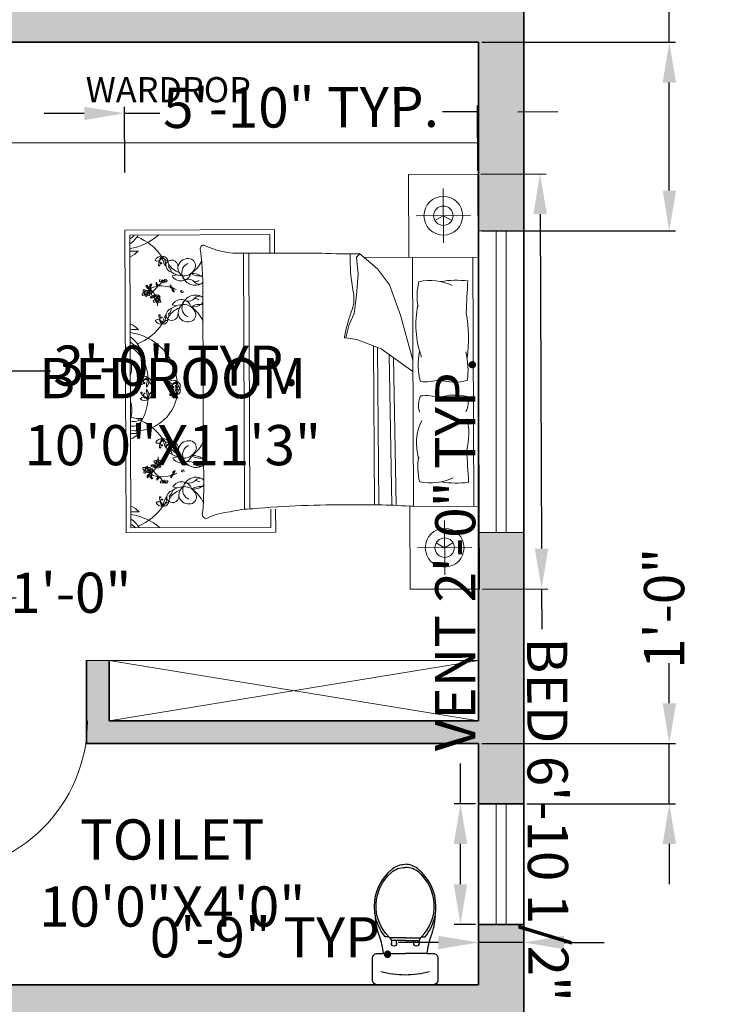
# Model space of a CAD drawing. Units: inches. Extents: x 2408 to 5087, y 2429 to 5085.
# Tile 9 of 12: x 2723 to 2864, y 2619 to 2815. Entities that reach past the tile are written whole.
import ezdxf

# ---------------------------------------------------------------- set-up
doc = ezdxf.new("R2010")
doc.units = ezdxf.units.IN
for name, color, linetype, lineweight in [('A-ANNO-DIMS', 2, 'Continuous', 18), ('A-ANNO-TEXT', 6, 'Continuous', 18), ('A-AREA-IDEN', 6, 'Continuous', 18), ('A-DOOR', 3, 'Continuous', 18), ('A-FLOR-CASE', 8, 'Continuous', 18), ('A-FLOR-FIXT', 9, 'Continuous', 18), ('A-FURN', 72, 'Continuous', 18), ('A-GLAZ', 4, 'Continuous', 18), ('A-WALL', 7, 'Continuous', 35), ('A-WALL-PATT', 252, 'Continuous', 13)]:
    doc.layers.add(name, color=color, linetype=linetype, lineweight=lineweight)
doc.layers.add('WC-Detail_dwgmodels.com', color=251, linetype='Continuous')
doc.layers.add('WC-Outline_dwgmodels.com', color=250, linetype='Continuous')
doc.styles.get("Standard").update_dxf_attribs({"font": 'arial.ttf'})
doc.dimstyles.new('ISO-25', dxfattribs={"dimtxt": 8, "dimasz": 8, "dimexe": 1.25, "dimexo": 0.625, "dimtad": 0, "dimdec": 1, "dimlunit": 4, "dimtxsty": 'Standard', "dimcen": 2.5, "dimadec": 0, "dimazin": 0, "dimtfac": 1, "dimtdec": 1, "dimtmove": 0, "dimatfit": 3, "dimfxl": 1, "dimarcsym": 0})

# ---------------------------------------------------------------- blocks, each defined once
blk = doc.blocks.new('door')
blk.add_lwpolyline([(2353.25, 2862.23), (2353.25, 2898.06), (2351.47, 2898.06), (2351.47, 2862.23), (2353.25, 2862.23)])
blk.add_arc((2353.25, 2862.23), 35.83, 90, 180)
blk = doc.blocks.new('bed')
for p, q in [((2542.13, 3205.85), (2660.24, 3205.85)), ((2553.94, 3188.29), (2553.94, 3203.72)), ((2565.75, 3205.85), (2565.75, 3173.43)), ((2636.62, 3204.33), (2565.75, 3204.33)), ((2648.43, 3188.29), (2648.43, 3203.72)), ((2561.66, 3196.01), (2546.23, 3196.01)), ((2640.72, 3196.01), (2656.15, 3196.01)), ((2565.75, 3187.18), (2636.62, 3187.18)), ((2582.16, 3183.67), (2595.04, 3187.18)), ((2598.2, 3187.18), (2591.73, 3178.18)), ((2573.55, 3180.57), (2582.16, 3183.67)), ((2636.26, 3181.07), (2593.37, 3180.46)), ((2636.3, 3182.28), (2594.25, 3181.69)), ((2569, 3177.22), (2573.55, 3180.57)), ((2591.73, 3178.18), (2589.1, 3171.24)), ((2564.7, 3172.2), (2569, 3177.22)), ((2636.2, 3176.13), (2590.88, 3175.95)), ((2636.2, 3177.35), (2591.35, 3177.17)), ((2565.65, 3171.24), (2564.7, 3172.2)), ((2570.44, 3171.72), (2565.65, 3171.24)), ((2576.42, 3171.24), (2570.44, 3171.72)), ((2581.68, 3170.52), (2576.42, 3171.24)), ((2584.79, 3169.09), (2581.68, 3170.52)), ((2589.1, 3171.24), (2588.62, 3168.13)), ((2588.62, 3168.13), (2584.79, 3169.09)), ((2557.72, 3147.95), (2564.4, 3147.95)), ((2557.72, 3105.4), (2557.72, 3147.95)), ((2637.28, 3147.95), (2643.83, 3147.95)), ((2643.83, 3147.95), (2643.83, 3105.4)), ((2564.4, 3146.58), (2559.09, 3146.58)), ((2559.09, 3146.58), (2559.09, 3106.77)), ((2642.46, 3146.58), (2637.25, 3146.58)), ((2642.46, 3106.77), (2642.46, 3146.58)), ((2637.16, 3140.58), (2564.39, 3140.58)), ((2637.27, 3139.11), (2564.39, 3139.11)), ((2625.17, 3127.51), (2577.21, 3127.51)), ((2570.73, 3118.75), (2570.47, 3120.08)), ((2578.98, 3118.75), (2579.25, 3120.08)), ((2622.57, 3118.75), (2622.31, 3120.08)), ((2630.82, 3118.75), (2631.08, 3120.08)), ((2643.83, 3105.4), (2557.72, 3105.4)), ((2559.09, 3106.77), (2642.46, 3106.77))]:
    blk.add_line(p, q)
for points in [[(2565.75, 3186.16), (2542.13, 3186.16), (2542.13, 3205.85)], [(2636.62, 3205.85), (2636.62, 3186.16), (2660.24, 3186.16), (2660.24, 3205.85)], [(2553.94, 3196.01), (2555.32, 3198.39)], [(2648.43, 3196.01), (2647.05, 3198.39)], [(2553.94, 3196.01), (2555.32, 3193.62)], [(2648.43, 3196.01), (2647.05, 3193.62)]]:
    blk.add_lwpolyline(points)
for points in [[(2572.54, 3202.91, 0.074897), (2572.68, 3195.19, -0.472817)], [(2600.63, 3194.76, 0.14099), (2600.87, 3202.63, 0.235245)], [(2605.68, 3194.76, -0.14099), (2605.44, 3202.63, -0.235245)], [(2629.84, 3202.91, -0.074897), (2629.69, 3195.19, 0.472817)], [(2564.45, 3161.38, 0.001242), (2564.39, 3138.97, -0.127202), (2562.03, 3127.8)], [(2637.13, 3141.51, 0.056112), (2637.98, 3135.02, 0.095341), (2639.64, 3128.76)]]:
    blk.add_lwpolyline(points, format="xyb")
for centre, radius in [((2553.94, 3196.01), 5.51), ((2648.43, 3196.01), 5.51), ((2553.94, 3196.01), 2.76), ((2648.43, 3196.01), 2.76), ((2577.55, 3114.47), 0.301), ((2624, 3114.47), 0.301), ((2575.59, 3111.3), 0.301), ((2625.97, 3111.3), 0.301)]:
    blk.add_circle(centre, radius)
for centre, radius, start, end in [((2637.64, 4326.92), 1125.9, 266.68521, 267.14978), ((2588.72, 3160.17), 42.84, 82.2196, 99.497), ((2597.77, 3181.81), 21.05, 81.5249, 103.96), ((2607.06, 3197.02), 5.84, 63.3437, 106.1026), ((2615.82, 3182.24), 20.76, 76.3427, 101.1841), ((2564.74, 4326.92), 1125.9, 272.85022, 273.31479), ((2587.59, 3192.09), 15.22, 155.1316, 191.7583), ((2614.79, 3192.09), 15.22, 348.2417, 24.8684), ((2586.71, 3190.81), 14.47, 354.0129, 15.8293), ((2619.6, 3190.81), 14.47, 164.1707, 185.9871), ((2585.08, 3215.54), 27.45, 258.0397, 289.2615), ((2596.2, 3209.54), 20.83, 259.8617, 283.6238), ((2607.85, 3194.98), 6.26, 245.0183, 288.5407), ((2618.79, 3203.12), 15.03, 243.8761, 286.1746), ((2576.75, 3204.29), 15.83, 255.1039, 281.0369), ((2625.62, 3204.29), 15.83, 258.9631, 284.8961), ((2848.35, 3172.75), 212.22, 176.1, 180.9282), ((2456.4, 3169.26), 108.33, 355.8294, 1.553), ((2566.72, 3214.02), 44.58, 267.4519, 281.3392), ((2577.37, 3160.89), 9.61, 66.2616, 101.3392), ((2596.82, 3212.77), 45.8, 250.1194, 259.3383), ((2588.35, 3168.04), 0.285, 268.8623, 19.7536), ((2912.96, 3165.03), 276.84, 179.1145, 184.8735), ((2563.11, 3127.88), 1.09, 183.98, 297.3412), ((2575.8, 3004.56), 122.95, 89.3433, 95.6887), ((2571.99, 3126.2), 1.42, 120.0293, 142.325), ((2571.99, 3126.2), 1.42, 44.4517, 63.558), ((2577.72, 3126.2), 1.42, 113.229, 135.5483), ((2577.72, 3126.2), 1.42, 37.675, 66.7144), ((2583.78, 3126.64), 4.89, 169.7133, 211.1782), ((2587.06, 3119.19), 8.94, 111.4941, 146.3329), ((2614.49, 3119.19), 8.94, 33.6671, 68.5059), ((2617.77, 3126.64), 4.89, 328.8218, 10.2867), ((2623.83, 3126.2), 1.42, 113.2856, 142.325), ((2623.83, 3126.2), 1.42, 44.4517, 66.7144), ((2628.78, 3012.64), 114.93, 85.2402, 91.8035), ((2629.56, 3126.2), 1.42, 106.6343, 135.5483), ((2629.56, 3126.2), 1.42, 37.675, 72.5814), ((2635.62, 3126.64), 4.89, 169.249, 211.1782), ((2638.75, 3128.16), 1.08, 246.5219, 33.8264), ((2567.86, 3123.48), 1.99, 84.4856, 181.0538), ((2562.65, 3119.19), 8.94, 33.6671, 63.2997), ((2567.25, 3122.01), 3.55, 355.2933, 76.921), ((2574.63, 3124.51), 4.56, 145.785, 184.7304), ((2565.93, 3126.64), 4.89, 328.8218, 9.1554), ((2569.72, 3125.36), 3.76, 289.2822, 29.1751), ((2574.17, 3123.35), 2.42, 131.5653, 195.1471), ((2569.15, 3124.68), 3.4, 7.436, 29.9149), ((2571.39, 3126.49), 1.77, 311.5653, 23.8354), ((2579.99, 3125.36), 3.76, 150.8249, 250.7178), ((2578.32, 3126.49), 1.77, 156.1646, 228.4347), ((2575.54, 3123.35), 2.42, 344.8529, 48.4347), ((2580.56, 3124.68), 3.4, 150.0851, 172.564), ((2575.08, 3124.51), 4.56, 355.2696, 34.215), ((2582.47, 3122.01), 3.55, 103.079, 184.7067), ((2581.85, 3123.48), 1.99, 358.9462, 95.5144), ((2619.7, 3123.48), 1.99, 84.4856, 181.0538), ((2619.08, 3122.01), 3.55, 355.2933, 76.921), ((2626.47, 3124.51), 4.56, 145.785, 184.7304), ((2621.56, 3125.36), 3.76, 289.2822, 29.1751), ((2626.01, 3123.35), 2.42, 131.5653, 195.1471), ((2620.99, 3124.68), 3.4, 7.436, 29.9149), ((2623.23, 3126.49), 1.77, 311.5653, 23.8354), ((2631.83, 3125.36), 3.76, 150.8249, 250.7178), ((2630.16, 3126.49), 1.77, 156.1646, 228.4347), ((2627.38, 3123.35), 2.42, 344.8529, 48.4347), ((2632.4, 3124.68), 3.4, 150.0851, 172.564), ((2626.92, 3124.51), 4.56, 355.2696, 34.215), ((2634.3, 3122.01), 3.55, 103.079, 184.7067), ((2638.9, 3119.19), 8.94, 113.6453, 146.3329), ((2633.69, 3123.48), 1.99, 358.9462, 95.5144), ((2568.68, 3123.2), 2.82, 174.9449, 262.8857), ((2569.79, 3124.27), 2.74, 201.5819, 291.4221), ((2569.27, 3121.29), 2.94, 299.9085, 73.1337), ((2574.63, 3124.51), 4.56, 212.7011, 216.3445), ((2571.13, 3122.53), 0.733, 257.3041, 15.1471), ((2575.17, 3121.56), 0.37, 280.4384, 100.4136), ((2580.45, 3121.29), 2.94, 106.8663, 240.0915), ((2578.59, 3122.53), 0.733, 164.8529, 282.6959), ((2575.08, 3124.51), 4.56, 323.6555, 327.2989), ((2579.93, 3124.27), 2.74, 248.5779, 338.4181), ((2581.04, 3123.2), 2.82, 277.1143, 5.0551), ((2620.51, 3123.2), 2.82, 174.9449, 262.8857), ((2621.62, 3124.27), 2.74, 201.5819, 291.4221), ((2621.1, 3121.29), 2.94, 299.9085, 73.1337), ((2626.47, 3124.51), 4.56, 212.7011, 216.3445), ((2622.96, 3122.53), 0.733, 257.3041, 15.1471), ((2626.38, 3121.56), 0.37, 79.5864, 259.5616), ((2632.29, 3121.29), 2.94, 106.8663, 240.0915), ((2630.43, 3122.53), 0.733, 164.8529, 282.6959), ((2626.92, 3124.51), 4.56, 323.6555, 327.2989), ((2631.76, 3124.27), 2.74, 248.5779, 338.4181), ((2632.87, 3123.2), 2.82, 277.1143, 5.0551), ((2568.03, 3118.65), 1.77, 80.264, 250.8688), ((2564.51, 3122.55), 5.58, 301.2614, 341.7045), ((2568.19, 3123.83), 3.43, 272.3591, 324.0401), ((2564.46, 3122.1), 6.34, 326.2883, 356.5076), ((2583.38, 3115.47), 9.78, 153.0032, 159.8941), ((2574.57, 3118.82), 0.241, 84.3784, 186.0543), ((2574.08, 3120.88), 1.9, 285.5129, 293.6099), ((2575.32, 3118.75), 0.62, 87.3579, 140.4944), ((2573.89, 3120.53), 1.87, 301.164, 321.5612), ((2575.2, 3121.41), 0.228, 102.7051, 280.4384), ((2572.37, 3120.86), 3.33, 324.6898, 333.4936), ((2581.53, 3123.83), 3.43, 215.9599, 267.6409), ((2585.25, 3122.1), 6.34, 183.4924, 213.7117), ((2585.2, 3122.55), 5.58, 198.2955, 238.7386), ((2581.69, 3118.65), 1.77, 289.1312, 99.736), ((2602.11, 3104.69), 15.42, 94.4623, 172.255), ((2602.17, 3118.92), 1.71, 137.7873, 219.1145), ((2600.23, 3118.97), 1.29, 298.5391, 58.3627), ((2602.13, 3119.71), 1.28, 63.0274, 163.8037), ((2600.84, 3122.7), 2.63, 271.4585, 315.3727), ((2601.91, 3117.85), 2.44, 45.5411, 114.3101), ((2604.13, 3130.37), 10.79, 252.593, 267.2582), ((2602.17, 3120.02), 1.26, 177.7585, 283.852), ((2604.6, 3121.34), 3.9, 198.9159, 238.011), ((2603.58, 3117.85), 2.44, 65.6899, 134.4589), ((2601.35, 3130.37), 10.79, 272.7418, 287.407), ((2602.43, 3118.96), 0.167, 283.852, 219.9245), ((2603.35, 3119.71), 1.28, 16.1963, 116.9726), ((2604.65, 3122.7), 2.63, 224.6273, 268.5415), ((2603.04, 3119.02), 0.101, 320.1909, 256.0209), ((2600.89, 3121.34), 3.9, 301.989, 341.0841), ((2603.32, 3120.02), 1.26, 256.148, 2.2415), ((2605.26, 3118.97), 1.29, 121.6373, 241.4609), ((2603.32, 3118.92), 1.71, 320.8855, 42.2127), ((2602.88, 3108.26), 11.94, 352.8636, 81.8197), ((2619.87, 3118.65), 1.77, 80.264, 250.8688), ((2616.35, 3122.55), 5.58, 301.2614, 341.7045), ((2620.02, 3123.83), 3.43, 272.3591, 324.0401), ((2616.3, 3122.1), 6.34, 326.2883, 356.5076), ((2627.67, 3120.53), 1.87, 218.4388, 238.836), ((2626.23, 3118.75), 0.62, 39.5056, 92.6421), ((2629.18, 3120.86), 3.33, 206.5064, 215.3102), ((2626.36, 3121.41), 0.228, 259.5616, 77.2949), ((2627.47, 3120.88), 1.9, 246.3901, 254.4871), ((2618.17, 3115.47), 9.78, 20.1059, 26.9968), ((2626.99, 3118.82), 0.241, 353.9457, 95.6216), ((2633.36, 3123.83), 3.43, 215.9599, 267.6409), ((2637.09, 3122.1), 6.34, 183.4924, 213.7117), ((2637.04, 3122.55), 5.58, 198.2955, 238.7386), ((2633.52, 3118.65), 1.77, 289.1312, 99.736), ((2566.53, 3116.2), 1.28, 92.9516, 193.728), ((2563.91, 3118.15), 2.63, 301.3827, 345.2969), ((2567.26, 3114.47), 2.44, 75.4653, 144.2343), ((2562.95, 3126.43), 10.79, 282.5173, 297.1824), ((2567.66, 3116.73), 1.09, 63.9755, 143.2681), ((2567.6, 3119.18), 2.21, 265.969, 344.3045), ((2569.99, 3116.24), 2.36, 96.1662, 141.5825), ((2572.14, 3116.72), 0.502, 101.5637, 142.6358), ((2571.72, 3116.26), 0.301, 273.2768, 86.7232), ((2572.07, 3116.54), 0.287, 91.1081, 181.8675), ((2572.38, 3115.96), 0.622, 80.3487, 133.6538), ((2571.74, 3117.11), 0.723, 288.7263, 352.5032), ((2572.26, 3115.32), 0.985, 83.0852, 105.7171), ((2572.23, 3117.08), 0.232, 345.2356, 144.9248), ((2572.44, 3116.32), 0.259, 317.6792, 80.3487), ((2573.89, 3117.9), 0.62, 101.3256, 154.4621), ((2573, 3120), 1.87, 280.2588, 300.656), ((2573.43, 3121.49), 3.33, 268.3264, 277.1302), ((2583.38, 3115.47), 9.78, 163.5842, 183.8277), ((2572.6, 3120), 1.9, 308.2101, 316.3071), ((2573.76, 3118.75), 0.567, 278.3432, 4.2869), ((2573.45, 3119.25), 0.99, 300.656, 332.6341), ((2574.19, 3118.59), 0.241, 55.7657, 157.4417), ((2574.34, 3119.78), 0.99, 269.1859, 301.164), ((2574.63, 3119.27), 0.567, 237.5332, 323.4768), ((2579.73, 3116.24), 2.36, 38.4175, 83.8338), ((2582.11, 3119.18), 2.21, 195.6955, 274.031), ((2582.05, 3116.73), 1.09, 36.7319, 116.0245), ((2582.45, 3114.47), 2.44, 35.7657, 104.5347), ((2586.77, 3126.43), 10.79, 242.8176, 257.4827), ((2583.19, 3116.2), 1.28, 346.272, 87.0484), ((2585.8, 3118.15), 2.63, 194.7031, 238.6173), ((2602.63, 3118.19), 0.192, 238.011, 71.5592), ((2602.66, 3118.28), 0.093, 71.5592, 188.0167), ((2602.86, 3118.19), 0.192, 108.4408, 301.989), ((2602.83, 3118.28), 0.093, 351.9833, 108.4408), ((2618.36, 3116.2), 1.28, 92.9516, 193.728), ((2615.75, 3118.15), 2.63, 301.3827, 345.2969), ((2619.1, 3114.47), 2.44, 75.4653, 144.2343), ((2614.78, 3126.43), 10.79, 282.5173, 297.1824), ((2619.5, 3116.73), 1.09, 63.9755, 143.2681), ((2619.44, 3119.18), 2.21, 265.969, 344.3045), ((2621.82, 3116.24), 2.36, 96.1662, 141.5825), ((2626.92, 3119.27), 0.567, 216.5232, 302.4668), ((2627.21, 3119.78), 0.99, 238.836, 270.8141), ((2627.79, 3118.75), 0.567, 175.7131, 261.6568), ((2627.36, 3118.59), 0.241, 22.5583, 124.2343), ((2628.1, 3119.25), 0.99, 207.3659, 239.344), ((2618.17, 3115.47), 9.78, 356.1723, 16.4158), ((2628.96, 3120), 1.9, 223.6929, 231.7899), ((2628.55, 3120), 1.87, 239.344, 259.7412), ((2628.12, 3121.49), 3.33, 262.8698, 271.6736), ((2627.66, 3117.9), 0.62, 25.5379, 78.6744), ((2629.11, 3116.32), 0.259, 99.6513, 222.3208), ((2629.17, 3115.96), 0.622, 46.3462, 99.6513), ((2629.32, 3117.08), 0.232, 35.0752, 194.7644), ((2629.82, 3117.11), 0.723, 187.4968, 251.2737), ((2629.29, 3115.32), 0.985, 74.2829, 96.9148), ((2629.48, 3116.54), 0.287, 358.1325, 88.8919), ((2629.41, 3116.72), 0.502, 37.3642, 78.4363), ((2629.83, 3116.26), 0.301, 93.2768, 266.7232), ((2633.95, 3119.18), 2.21, 195.6955, 274.031), ((2631.56, 3116.24), 2.36, 38.4175, 83.8338), ((2633.89, 3116.73), 1.09, 36.7319, 116.0245), ((2634.29, 3114.47), 2.44, 35.7657, 104.5347), ((2638.61, 3126.43), 10.79, 242.8176, 257.4827), ((2637.64, 3118.15), 2.63, 194.7031, 238.6173), ((2635.02, 3116.2), 1.28, 346.272, 87.0484), ((2547.61, 3104.69), 15.42, 7.745, 41.8856), ((2574, 3103.17), 15.42, 124.3865, 158.5908), ((2566.96, 3115.53), 1.71, 167.7115, 249.0387), ((2565.25, 3114.61), 1.29, 328.4633, 88.2869), ((2567.85, 3118.83), 3.9, 228.8402, 267.9352), ((2566.4, 3116.48), 1.26, 207.6827, 313.7762), ((2567.16, 3115.69), 0.167, 313.7762, 249.7183), ((2567.7, 3115.22), 0.093, 101.4834, 217.9409), ((2567.72, 3115.13), 0.192, 267.9352, 101.4834), ((2572.13, 3115.7), 0.497, 217.7621, 259.0403), ((2572.67, 3116.36), 0.913, 203.4276, 227.6104), ((2572.27, 3116.48), 0.492, 229.7889, 317.6792), ((2571.71, 3115.43), 0.699, 355.053, 68.3618), ((2572.18, 3115.39), 0.231, 232.4737, 355.053), ((2565.44, 3107.15), 11.21, 43.1541, 52.0459), ((2573.19, 3113.92), 0.62, 101.3256, 154.4621), ((2572.3, 3116.03), 1.87, 280.2588, 300.656), ((2572.73, 3117.52), 3.33, 268.3264, 277.1302), ((2571.89, 3116.02), 1.9, 308.2101, 316.3071), ((2573.06, 3114.77), 0.567, 278.3432, 4.2869), ((2572.74, 3115.27), 0.99, 300.656, 332.6341), ((2573.49, 3114.62), 0.241, 55.7657, 157.4417), ((2578.51, 3115.22), 4.9, 184.756, 209.2041), ((2585.57, 3125.67), 16.14, 222.2412, 232.1744), ((2579.01, 3108.71), 5.88, 120.544, 139.818), ((2575.98, 3114.61), 0.833, 272.8499, 356.1226), ((2575.25, 3114.91), 1.37, 304.5369, 16.3699), ((2575.39, 3114.28), 0.807, 321.7607, 7.9252), ((2575.56, 3113.13), 0.807, 8.7227, 54.8872), ((2575.61, 3112.48), 1.37, 0.278, 72.111), ((2577.15, 3114.53), 0.97, 127.3105, 187.9252), ((2576.22, 3112.98), 0.833, 20.5253, 88.5375), ((2575.82, 3114.64), 0.996, 355.0106, 41.658), ((2576.92, 3113.9), 0.298, 148.0499, 225.6268), ((2579.01, 3108.71), 5.88, 113.0501, 113.8477), ((2577.47, 3113.56), 0.948, 104.7558, 148.0499), ((2576.94, 3114.24), 0.594, 247.4086, 351.4386), ((2577.22, 3114.89), 0.41, 126.1046, 271.4281), ((2577.18, 3115), 0.295, 353.7526, 131.7054), ((2577.11, 3114.21), 0.199, 262.906, 7.132), ((2576.9, 3114.65), 0.414, 0.0645, 61.1507), ((2577, 3115), 0.473, 311.8413, 355.7877), ((2577.97, 3114.93), 0.502, 101.5637, 176.365), ((2577.96, 3113.91), 0.497, 151.2196, 259.0403), ((2577.9, 3114.75), 0.287, 91.1081, 181.8675), ((2578.5, 3114.57), 0.913, 203.4276, 227.6104), ((2578.21, 3114.17), 0.622, 80.3487, 133.6538), ((2578.1, 3114.69), 0.492, 229.7889, 317.6792), ((2577.57, 3115.33), 0.723, 288.7263, 352.5032), ((2577.54, 3113.65), 0.699, 355.053, 68.3618), ((2578.09, 3113.53), 0.985, 83.0852, 105.7171), ((2578.06, 3115.29), 0.232, 345.2356, 144.9248), ((2578.01, 3113.61), 0.231, 232.4737, 355.053), ((2578.27, 3114.53), 0.259, 317.6792, 80.3487), ((2579.01, 3108.71), 5.88, 87.1071, 94.7585), ((2582, 3115.13), 0.192, 78.5166, 272.0648), ((2581.86, 3118.83), 3.9, 272.0648, 311.1598), ((2582.02, 3115.22), 0.093, 322.0591, 78.5166), ((2583.31, 3116.48), 1.26, 226.2238, 332.3173), ((2582.57, 3115.76), 0.101, 290.2667, 226.2271), ((2584.47, 3114.61), 1.29, 91.7131, 211.5367), ((2582.76, 3115.53), 1.71, 290.9613, 12.2885), ((2575.72, 3103.17), 15.42, 21.4092, 55.6135), ((2625.83, 3103.17), 15.42, 124.3865, 158.5908), ((2618.79, 3115.53), 1.71, 167.7115, 249.0387), ((2618.24, 3116.48), 1.26, 207.6827, 313.7762), ((2619.69, 3118.83), 3.9, 228.8402, 267.9352), ((2617.08, 3114.61), 1.29, 328.4633, 88.2869), ((2619, 3115.69), 0.167, 313.7762, 249.7183), ((2619.54, 3115.22), 0.093, 101.4834, 217.9409), ((2619.56, 3115.13), 0.192, 267.9352, 101.4834), ((2622.54, 3108.71), 5.88, 85.2415, 92.8929), ((2623.28, 3114.53), 0.259, 99.6513, 222.3208), ((2623.45, 3114.69), 0.492, 222.3208, 310.2111), ((2623.34, 3114.17), 0.622, 46.3462, 99.6513), ((2623.49, 3115.29), 0.232, 35.0752, 194.7644), ((2623.98, 3115.33), 0.723, 187.4968, 251.2737), ((2624.01, 3113.65), 0.699, 111.6382, 184.947), ((2623.54, 3113.61), 0.231, 184.947, 307.5263), ((2623.46, 3113.53), 0.985, 74.2829, 96.9148), ((2623.65, 3114.75), 0.287, 358.1325, 88.8919), ((2623.05, 3114.57), 0.913, 312.3896, 336.5724), ((2623.58, 3114.93), 0.502, 3.635, 78.4363), ((2623.59, 3113.91), 0.497, 280.9597, 28.7804), ((2624.61, 3114.24), 0.594, 188.5614, 292.5914), ((2624.38, 3115), 0.295, 48.2946, 186.2474), ((2624.55, 3115), 0.473, 184.2123, 228.1587), ((2624.65, 3114.65), 0.414, 118.8493, 179.9355), ((2624.44, 3114.21), 0.199, 172.868, 277.094), ((2624.33, 3114.89), 0.41, 268.5719, 53.8954), ((2624.08, 3113.56), 0.948, 31.9501, 75.2442), ((2625.33, 3112.98), 0.833, 91.4625, 159.4747), ((2625.94, 3112.48), 1.37, 107.889, 179.722), ((2625.73, 3114.64), 0.996, 138.342, 184.9894), ((2625.57, 3114.61), 0.833, 183.8774, 267.1501), ((2622.54, 3108.71), 5.88, 66.1523, 66.9499), ((2624.63, 3113.9), 0.298, 314.3732, 31.9501), ((2626.3, 3114.91), 1.37, 163.6301, 235.4631), ((2624.4, 3114.53), 0.97, 352.0748, 52.6895), ((2625.99, 3113.13), 0.807, 125.1128, 171.2773), ((2626.16, 3114.28), 0.807, 172.0748, 218.2393), ((2622.54, 3108.71), 5.88, 40.182, 59.456), ((2615.98, 3125.67), 16.14, 307.8256, 317.7588), ((2623.04, 3115.22), 4.9, 330.7959, 355.244), ((2636.11, 3107.15), 11.21, 127.9541, 136.8459), ((2628.06, 3114.62), 0.241, 22.5583, 124.2343), ((2628.49, 3114.77), 0.567, 175.7131, 261.6568), ((2628.81, 3115.27), 0.99, 207.3659, 239.344), ((2629.66, 3116.02), 1.9, 223.6929, 231.7899), ((2629.26, 3116.03), 1.87, 239.344, 259.7412), ((2628.83, 3117.52), 3.33, 262.8698, 271.6736), ((2628.36, 3113.92), 0.62, 25.5379, 78.6744), ((2629.29, 3116.48), 0.492, 222.3208, 310.2111), ((2629.84, 3115.43), 0.699, 111.6382, 184.947), ((2629.37, 3115.39), 0.231, 184.947, 307.5263), ((2628.88, 3116.36), 0.913, 312.3896, 336.5724), ((2629.42, 3115.7), 0.497, 280.9597, 322.2379), ((2633.83, 3115.13), 0.192, 78.5166, 272.0648), ((2633.7, 3118.83), 3.9, 272.0648, 311.1598), ((2633.85, 3115.22), 0.093, 322.0591, 78.5166), ((2635.15, 3116.48), 1.26, 226.2238, 332.3173), ((2634.41, 3115.76), 0.101, 290.2667, 226.2271), ((2636.31, 3114.61), 1.29, 91.7131, 211.5367), ((2634.6, 3115.53), 1.71, 290.9613, 12.2885), ((2627.56, 3103.17), 15.42, 21.4092, 55.6135), ((2653.94, 3104.69), 15.42, 138.1144, 172.255), ((2573.4, 3112.83), 0.336, 146.8636, 236.9021), ((2578.13, 3120.23), 8.79, 235.1882, 238.8844), ((2573.97, 3113.32), 0.909, 199.4799, 267.6828), ((2573.87, 3112.98), 0.783, 212.8155, 277.3992), ((2573.42, 3112.45), 0.909, 266.9701, 338.2913), ((2568.62, 3118.94), 8.79, 302.6784, 306.3746), ((2573.65, 3111.74), 0.336, 214.3538, 304.3923), ((2573.77, 3113.01), 0.348, 238.8844, 314.2646), ((2573.7, 3112.23), 0.783, 280.3057, 17.1958), ((2573.63, 3112.15), 0.348, 306.3746, 21.7548), ((2574.2, 3112.37), 0.262, 19.3605, 201.7548), ((2574.2, 3112.57), 0.262, 311.8703, 134.2646), ((2579.13, 3110.18), 5.24, 153.7819, 158.2913), ((2574.96, 3113.76), 1.37, 247.2305, 319.0635), ((2574.51, 3113.3), 0.807, 264.4544, 310.6188), ((2578.51, 3115.22), 4.9, 214.0033, 222.4917), ((2575.1, 3112.98), 0.833, 218.3208, 298.8162), ((2574.95, 3110.73), 0.298, 148.0499, 225.6268), ((2575.51, 3110.39), 0.948, 104.7558, 148.0499), ((2574.97, 3111.07), 0.594, 247.4086, 351.4386), ((2575.25, 3111.72), 0.41, 126.1046, 271.4281), ((2575.21, 3111.83), 0.295, 353.7526, 131.7054), ((2575.66, 3111.95), 0.97, 70.0041, 130.6188), ((2575.14, 3111.04), 0.199, 262.906, 7.132), ((2574.93, 3111.48), 0.414, 0.0645, 61.1507), ((2575.03, 3111.83), 0.473, 311.8413, 355.7877), ((2575.04, 3113.13), 0.996, 297.7043, 344.3516), ((2576, 3111.76), 0.502, 101.5637, 176.365), ((2576, 3110.74), 0.497, 151.2196, 259.0403), ((2575.94, 3111.58), 0.287, 91.1081, 181.8675), ((2576.53, 3111.4), 0.913, 203.4276, 227.6104), ((2576.24, 3111), 0.622, 80.3487, 133.6538), ((2576.13, 3111.52), 0.492, 229.7889, 317.6792), ((2575.6, 3112.16), 0.723, 288.7263, 352.5032), ((2575.58, 3110.48), 0.699, 355.053, 68.3618), ((2576.12, 3110.36), 0.985, 83.0852, 105.7171), ((2576.09, 3112.12), 0.232, 345.2356, 144.9248), ((2576.3, 3111.36), 0.259, 317.6792, 80.3487), ((2577.32, 3113.39), 0.97, 188.7227, 249.3375), ((2576.08, 3112.91), 0.996, 334.9899, 21.6373), ((2600.93, 3096.43), 15.42, 94.4623, 117.4146), ((2600.99, 3110.66), 1.71, 137.7873, 219.1145), ((2599.05, 3110.71), 1.29, 298.5391, 58.3627), ((2600.99, 3111.76), 1.26, 177.7585, 283.852), ((2600.95, 3111.45), 1.28, 63.0274, 163.8037), ((2599.66, 3114.44), 2.63, 271.4585, 315.3727), ((2600.73, 3109.59), 2.44, 45.5411, 114.3101), ((2603.42, 3113.07), 3.9, 198.9159, 238.011), ((2602.95, 3122.11), 10.79, 252.593, 267.2582), ((2601.25, 3110.7), 0.167, 283.852, 219.9245), ((2604.76, 3109.59), 2.44, 65.6899, 134.4589), ((2602.54, 3122.11), 10.79, 272.7418, 287.407), ((2604.54, 3111.45), 1.28, 16.1963, 116.9726), ((2605.83, 3114.44), 2.63, 224.6273, 268.5415), ((2604.22, 3110.76), 0.101, 320.1909, 256.0209), ((2602.07, 3113.07), 3.9, 301.989, 341.0841), ((2604.5, 3111.76), 1.26, 256.148, 2.2415), ((2606.44, 3110.71), 1.29, 121.6373, 241.4609), ((2604.5, 3110.66), 1.71, 320.8855, 42.2127), ((2604.56, 3096.43), 15.42, 62.5854, 85.5377), ((2625.48, 3112.91), 0.996, 158.3627, 205.0101), ((2624.23, 3113.39), 0.97, 290.6625, 351.2773), ((2625.25, 3111.36), 0.259, 99.6513, 222.3208), ((2625.42, 3111.52), 0.492, 222.3208, 310.2111), ((2625.31, 3111), 0.622, 46.3462, 99.6513), ((2625.46, 3112.12), 0.232, 35.0752, 194.7644), ((2625.95, 3112.16), 0.723, 187.4968, 251.2737), ((2625.98, 3110.48), 0.699, 111.6382, 184.947), ((2625.43, 3110.36), 0.985, 74.2829, 96.9148), ((2625.89, 3111.95), 0.97, 49.3812, 109.9959), ((2626.59, 3113.76), 1.37, 220.9365, 292.7695), ((2626.52, 3113.13), 0.996, 195.6484, 242.2957), ((2625.62, 3111.58), 0.287, 358.1325, 88.8919), ((2625.02, 3111.4), 0.913, 312.3896, 336.5724), ((2625.55, 3111.76), 0.502, 3.635, 78.4363), ((2625.56, 3110.74), 0.497, 280.9597, 28.7804), ((2626.58, 3111.07), 0.594, 188.5614, 292.5914), ((2626.45, 3112.98), 0.833, 241.1838, 321.6792), ((2626.34, 3111.83), 0.295, 48.2946, 186.2474), ((2626.52, 3111.83), 0.473, 184.2123, 228.1587), ((2626.62, 3111.48), 0.414, 118.8493, 179.9355), ((2626.41, 3111.04), 0.199, 172.868, 277.094), ((2626.3, 3111.72), 0.41, 268.5719, 53.8954), ((2626.05, 3110.39), 0.948, 31.9501, 75.2442), ((2627.04, 3113.3), 0.807, 229.3812, 275.5456), ((2623.04, 3115.22), 4.9, 317.5083, 325.9967), ((2626.6, 3110.73), 0.298, 314.3732, 31.9501), ((2627.86, 3112.23), 0.783, 162.8042, 259.6943), ((2627.35, 3112.57), 0.262, 45.7354, 228.1297), ((2627.36, 3112.37), 0.262, 338.2452, 160.6395), ((2622.42, 3110.18), 5.24, 21.7087, 26.2181), ((2628.13, 3112.45), 0.909, 201.7087, 273.0299), ((2627.78, 3113.01), 0.348, 225.7354, 301.1156), ((2627.92, 3112.15), 0.348, 158.2452, 233.6254), ((2627.68, 3112.98), 0.783, 262.6008, 327.1845), ((2627.58, 3113.32), 0.909, 272.3172, 340.5201), ((2632.93, 3118.94), 8.79, 233.6254, 237.3216), ((2627.91, 3111.74), 0.336, 235.6077, 325.6462), ((2623.42, 3120.23), 8.79, 301.1156, 304.8118), ((2628.15, 3112.83), 0.336, 303.0979, 33.1364), ((2555.35, 3102.63), 7.52, 33.4617, 60.1116), ((2552.64, 3101.23), 9.37, 36.3036, 46.4814), ((2559.56, 3104.37), 6.27, 22.5547, 48.9546), ((2542.38, 3107.74), 21.34, 357.4081, 3.6519), ((2576.04, 3110.44), 0.231, 232.4737, 355.053), ((2590.16, 3104.37), 6.27, 131.0454, 157.4453), ((2607.34, 3107.74), 21.34, 176.3481, 182.5919), ((2594.37, 3102.63), 7.52, 91.272, 146.5383), ((2597.07, 3101.23), 9.37, 107.8504, 143.6964), ((2601.99, 3098.59), 13.93, 124.0123, 144.053), ((2601.45, 3109.93), 0.192, 238.011, 71.5592), ((2601.48, 3110.02), 0.093, 71.5592, 188.0167), ((2604.04, 3109.93), 0.192, 108.4408, 301.989), ((2604.01, 3110.02), 0.093, 351.9833, 108.4408), ((2604.43, 3109.35), 6.91, 338.117, 6.6195), ((2610.76, 3107.42), 2.77, 346.3898, 79.0739), ((2608.68, 3107.8), 3.5, 342.8609, 41.9049), ((2594.21, 3107.74), 21.34, 357.4081, 3.6519), ((2611.39, 3104.37), 6.27, 22.5547, 48.9546), ((2625.51, 3110.44), 0.231, 184.947, 307.5263), ((2642, 3104.37), 6.27, 131.0454, 157.4453), ((2659.17, 3107.74), 21.34, 176.3481, 182.5919), ((2646.21, 3102.63), 7.52, 119.8884, 146.5383), ((2648.91, 3101.23), 9.37, 133.5186, 143.6964), ((2596.61, 3098.66), 8.48, 73.5431, 107.0202), ((2599.97, 3094.29), 12.54, 94.3787, 95.6357), ((2606.58, 3085.7), 22.41, 109.7217, 109.9028), ((2608.88, 3098.66), 8.48, 72.9798, 106.4569), ((2605.52, 3094.29), 12.54, 84.3643, 85.6213), ((2598.91, 3085.7), 22.41, 70.0972, 70.2783)]:
    blk.add_arc(centre, radius, start, end)
blk = doc.blocks.new('pan')
at = {"layer": 'WC-Detail_dwgmodels.com'}
for p, q in [((2600.67, 3096.11), (2600.67, 3096.83)), ((2601.96, 3096.83), (2601.96, 3096.11)), ((2606.1, 3096.83), (2606.1, 3096.11)), ((2607.39, 3096.11), (2607.39, 3096.83)), ((2600.31, 3095.45), (2600.67, 3096.11)), ((2601.96, 3096.11), (2600.67, 3096.11)), ((2604.03, 3096.11), (2601.96, 3096.11)), ((2604.03, 3096.11), (2606.1, 3096.11)), ((2606.1, 3096.11), (2607.39, 3096.11)), ((2607.75, 3095.45), (2607.39, 3096.11))]:
    blk.add_line(p, q, dxfattribs=at)
for points in [[(2600.04, 3095.18, 0.434217), (2600.67, 3079.55, 0.182634), (2604.03, 3078.32, 2.693815)], [(2599.14, 3095.18, 0.094048), (2597.09, 3091.32, 0.16845)], [(2600.04, 3095.18), (2599.14, 3095.18, 0.416606)], [(2600.31, 3095.45, 0.008985), (2600.04, 3095.18, 0.182634)], [(2604.03, 3095.45), (2600.31, 3095.45, 0.008985)], [(2604.03, 3095.45), (2607.75, 3095.45, -0.444938)], [(2608.02, 3095.18, -0.434217), (2607.39, 3079.55, -0.182634), (2604.03, 3078.32, -2.693815)], [(2607.75, 3095.45, -0.008985), (2608.02, 3095.18, -0.182634)], [(2608.02, 3095.18), (2608.92, 3095.18, -0.416606)], [(2608.92, 3095.18, -0.105447), (2611.12, 3090.81, -0.16845)], [(2597.09, 3091.32, 0.026594), (2596.78, 3090.11, 0.16845)], [(2611.12, 3090.81, -0.015301), (2611.28, 3090.11, -0.16845)]]:
    blk.add_lwpolyline(points, format="xyb", dxfattribs=at)
for centre, radius, start, end in [((2604.04, 3081.23), 23.26, 90.028, 104.6712), ((2604.02, 3081.23), 23.26, 75.3288, 89.972), ((2601.32, 3096.83), 0.645, 0, 180), ((2606.74, 3096.83), 0.645, 0, 180)]:
    blk.add_arc(centre, radius, start, end, dxfattribs=at)
at = {"layer": 'WC-Outline_dwgmodels.com'}
for points in [[(2610.82, 3099.25, 0.414214), (2611.96, 3100.39), (2611.96, 3105.7, 0.414214), (2610.82, 3106.84), (2604.03, 3106.84), (2597.24, 3106.84, 0.414214), (2596.1, 3105.7), (2596.1, 3100.39, 0.414214), (2597.24, 3099.25), (2598.79, 3099.25, -0.052345), (2597.77, 3095.01, 0.071131), (2596.78, 3090.11, 0.160777)], [(2598.79, 3099.25), (2604.03, 3099.25, 0.414214)], [(2609.26, 3099.25), (2604.03, 3099.25, -0.414214)], [(2611.28, 3090.11, 0.071131), (2610.29, 3095.01, -0.052345), (2609.26, 3099.25), (2610.82, 3099.25, 0.414214)], [(2596.78, 3090.11, 0.048023), (2596.56, 3087.87, 0.16845)], [(2611.28, 3090.11, -0.048023), (2611.5, 3087.87, -0.16845)], [(2596.56, 3087.87, 0.230343), (2601.03, 3078.62, 0.16845), (2604.03, 3077.58, 2.883082)], [(2611.5, 3087.87, -0.230343), (2607.03, 3078.62, -0.16845), (2604.03, 3077.58, -2.883082)]]:
    blk.add_lwpolyline(points, format="xyb", dxfattribs=at)
blk = doc.blocks.new('WIN-60x9')
for p, q in [((3.5, 60), (3.5, 0)), ((5.5, 60), (5.5, 0))]:
    blk.add_line(p, q)
blk.add_lwpolyline([(0, 60), (9, 60), (9, 0), (0, 0)], close=True)
blk = doc.blocks.new('WIN-24x9')
for p, q in [((0, 5.5), (24, 5.5)), ((0, 3.5), (24, 3.5))]:
    blk.add_line(p, q)
blk.add_lwpolyline([(0, 9), (24, 9), (24, 0), (0, 0)], close=True)
blk = doc.blocks.new('*D35')
at = {"layer": 'A-ANNO-DIMS', "color": 0, "lineweight": -2, "transparency": 16777216}
for p, q in [((2810.89, 2658.55), (2810.89, 2666.55)), ((2813.87, 2658.55), (2809.64, 2658.55)), ((2810.89, 2642.55), (2810.89, 2650.55)), ((2813.87, 2634.55), (2809.64, 2634.55))]:
    blk.add_line(p, q, dxfattribs=at)
at = {"layer": 'A-ANNO-DIMS', "color": 0, "transparency": 16777216}
for points in [[(2809.56, 2650.55), (2812.23, 2650.55), (2810.89, 2658.55)], [(2809.56, 2642.55), (2812.23, 2642.55), (2810.89, 2634.55)]]:
    blk.add_solid(points, dxfattribs=at)
at = {"layer": 'Defpoints', "color": 0, "transparency": 16777216}
for p in [(2810.89, 2658.55), (2814.49, 2658.55), (2814.49, 2634.55)]:
    blk.add_point(p, dxfattribs=at)
at = {"layer": 'A-ANNO-DIMS', "color": 0, "transparency": 16777216, "insert": (2810.89, 2708.22), "char_height": 8, "attachment_point": 5, "rotation": 90}
blk.add_mtext('VENT 2\'-0" TYP.', dxfattribs=at)
blk = doc.blocks.new('*D36')
at = {"layer": 'A-ANNO-DIMS', "color": 0, "lineweight": -2, "transparency": 16777216}
for p, q in [((2814.49, 2633.93), (2814.49, 2629.7)), ((2823.49, 2633.93), (2823.49, 2629.7)), ((2806.49, 2630.95), (2798.49, 2630.95)), ((2823.49, 2630.95), (2814.49, 2630.95)), ((2831.49, 2630.95), (2839.49, 2630.95))]:
    blk.add_line(p, q, dxfattribs=at)
at = {"layer": 'A-ANNO-DIMS', "color": 0, "transparency": 16777216}
for points in [[(2806.49, 2632.29), (2806.49, 2629.62), (2814.49, 2630.95)], [(2831.49, 2632.29), (2831.49, 2629.62), (2823.49, 2630.95)]]:
    blk.add_solid(points, dxfattribs=at)
at = {"layer": 'Defpoints', "color": 0, "transparency": 16777216}
for p in [(2814.49, 2634.55), (2823.49, 2634.55), (2814.49, 2630.95)]:
    blk.add_point(p, dxfattribs=at)
at = {"layer": 'A-ANNO-DIMS', "color": 0, "transparency": 16777216, "insert": (2773.49, 2630.95), "char_height": 8, "attachment_point": 5}
blk.add_mtext('0\'-9" TYP.', dxfattribs=at)
blk = doc.blocks.new('*D38')
at = {"layer": 'A-ANNO-DIMS', "color": 0, "lineweight": -2, "transparency": 16777216}
for p, q in [((2685.49, 2749.43), (2685.49, 2743.43)), ((2721.31, 2749.43), (2721.31, 2743.43)), ((2693.49, 2744.68), (2713.31, 2744.68)), ((2721.31, 2744.68), (2729.31, 2744.68))]:
    blk.add_line(p, q, dxfattribs=at)
at = {"layer": 'A-ANNO-DIMS', "color": 0, "transparency": 16777216}
for points in [[(2693.49, 2746.02), (2693.49, 2743.35), (2685.49, 2744.68)], [(2713.31, 2746.02), (2713.31, 2743.35), (2721.31, 2744.68)]]:
    blk.add_solid(points, dxfattribs=at)
at = {"layer": 'Defpoints', "color": 0, "transparency": 16777216}
for p in [(2685.49, 2750.05), (2721.31, 2750.05), (2721.31, 2744.68)]:
    blk.add_point(p, dxfattribs=at)
at = {"layer": 'A-ANNO-DIMS', "color": 0, "transparency": 16777216, "insert": (2754.31, 2744.68), "char_height": 8, "attachment_point": 5}
blk.add_mtext('3\'-0" TYP.', dxfattribs=at)
blk = doc.blocks.new('*D43')
at = {"layer": 'A-ANNO-DIMS', "color": 0, "lineweight": -2, "transparency": 16777216}
for p, q in [((2814.95, 2783.84), (2827.96, 2783.89)), ((2826.75, 2775.89), (2827.01, 2709.32)), ((2815.28, 2701.27), (2828.29, 2701.33)), ((2827.04, 2701.32), (2827.07, 2693.32))]:
    blk.add_line(p, q, dxfattribs=at)
at = {"layer": 'A-ANNO-DIMS', "color": 0, "transparency": 16777216}
for points in [[(2828.08, 2775.89), (2825.41, 2775.88), (2826.71, 2783.89)], [(2828.34, 2709.33), (2825.68, 2709.32), (2827.04, 2701.32)]]:
    blk.add_solid(points, dxfattribs=at)
at = {"layer": 'Defpoints', "color": 0, "transparency": 16777216}
for p in [(2814.33, 2783.84), (2814.66, 2701.27), (2827.04, 2701.32)]:
    blk.add_point(p, dxfattribs=at)
at = {"layer": 'A-ANNO-DIMS', "color": 0, "transparency": 16777216, "insert": (2827.27, 2643.02), "char_height": 8, "attachment_point": 5, "rotation": 270.2276}
blk.add_mtext('BED 6\'-10 1/2" TYP.', dxfattribs=at)
blk = doc.blocks.new('*D44')
at = {"layer": 'A-ANNO-DIMS', "color": 0, "lineweight": -2, "transparency": 16777216}
for p, q in [((2736.06, 2795.91), (2728.06, 2795.88)), ((2744.11, 2784.18), (2744.06, 2797.19)), ((2744.06, 2795.94), (2751.06, 2795.97)), ((2814.28, 2796.22), (2807.29, 2796.19)), ((2814.33, 2784.46), (2814.28, 2797.47)), ((2822.28, 2796.25), (2830.28, 2796.29))]:
    blk.add_line(p, q, dxfattribs=at)
at = {"layer": 'A-ANNO-DIMS', "color": 0, "transparency": 16777216}
for points in [[(2822.28, 2797.59), (2822.29, 2794.92), (2814.28, 2796.22)], [(2736.06, 2797.24), (2736.07, 2794.58), (2744.06, 2795.94)]]:
    blk.add_solid(points, dxfattribs=at)
at = {"layer": 'Defpoints', "color": 0, "transparency": 16777216}
for p in [(2814.28, 2796.22), (2814.33, 2783.84), (2744.11, 2783.56)]:
    blk.add_point(p, dxfattribs=at)
at = {"layer": 'A-ANNO-DIMS', "color": 0, "transparency": 16777216, "insert": (2779.17, 2796.08), "char_height": 8, "attachment_point": 5, "rotation": 0.2276}
blk.add_mtext('5\'-10" TYP.', dxfattribs=at)
blk = doc.blocks.new('*D76')
at = {"layer": 'A-ANNO-DIMS', "color": 0, "lineweight": -2, "transparency": 16777216}
for p, q in [((2852.44, 2810.05), (2852.44, 2818.05)), ((2815.12, 2810.05), (2853.69, 2810.05)), ((2852.44, 2780.55), (2852.44, 2802.05)), ((2815.12, 2772.55), (2853.69, 2772.55))]:
    blk.add_line(p, q, dxfattribs=at)
at = {"layer": 'A-ANNO-DIMS', "color": 0, "transparency": 16777216}
for points in [[(2851.11, 2802.05), (2853.78, 2802.05), (2852.44, 2810.05)], [(2851.11, 2780.55), (2853.78, 2780.55), (2852.44, 2772.55)]]:
    blk.add_solid(points, dxfattribs=at)
at = {"layer": 'Defpoints', "color": 0, "transparency": 16777216}
for p in [(2814.49, 2810.05), (2852.44, 2810.05), (2814.49, 2772.55)]:
    blk.add_point(p, dxfattribs=at)
at = {"layer": 'A-ANNO-DIMS', "color": 0, "transparency": 16777216, "insert": (2852.44, 2838.63), "char_height": 8, "attachment_point": 5, "rotation": 90}
blk.add_mtext('3\'-1 1/2"', dxfattribs=at)
blk = doc.blocks.new('*D78')
at = {"layer": 'A-ANNO-DIMS', "color": 0, "lineweight": -2, "transparency": 16777216}
for p, q in [((2852.44, 2678.55), (2852.44, 2686.55)), ((2815.12, 2670.55), (2853.69, 2670.55)), ((2852.44, 2658.55), (2852.44, 2670.55)), ((2824.12, 2658.55), (2853.69, 2658.55)), ((2852.44, 2650.55), (2852.44, 2642.55))]:
    blk.add_line(p, q, dxfattribs=at)
at = {"layer": 'A-ANNO-DIMS', "color": 0, "transparency": 16777216}
for points in [[(2851.11, 2678.55), (2853.78, 2678.55), (2852.44, 2670.55)], [(2851.11, 2650.55), (2853.78, 2650.55), (2852.44, 2658.55)]]:
    blk.add_solid(points, dxfattribs=at)
at = {"layer": 'Defpoints', "color": 0, "transparency": 16777216}
for p in [(2814.49, 2670.55), (2852.44, 2670.55), (2823.49, 2658.55)]:
    blk.add_point(p, dxfattribs=at)
at = {"layer": 'A-ANNO-DIMS', "color": 0, "transparency": 16777216, "insert": (2852.44, 2697.44), "char_height": 8, "attachment_point": 5, "rotation": 90}
blk.add_mtext('1\'-0"', dxfattribs=at)
blk = doc.blocks.new('*D80')
at = {"layer": 'A-ANNO-DIMS', "color": 0, "lineweight": -2, "transparency": 16777216}
for p, q in [((2694.49, 2671.18), (2694.49, 2700.75)), ((2706.49, 2671.18), (2706.49, 2700.75)), ((2686.49, 2699.5), (2678.49, 2699.5)), ((2694.49, 2699.5), (2706.49, 2699.5)), ((2714.49, 2699.5), (2722.49, 2699.5))]:
    blk.add_line(p, q, dxfattribs=at)
at = {"layer": 'A-ANNO-DIMS', "color": 0, "transparency": 16777216}
for points in [[(2686.49, 2700.84), (2686.49, 2698.17), (2694.49, 2699.5)], [(2714.49, 2700.84), (2714.49, 2698.17), (2706.49, 2699.5)]]:
    blk.add_solid(points, dxfattribs=at)
at = {"layer": 'Defpoints', "color": 0, "transparency": 16777216}
for p in [(2706.49, 2699.5), (2694.49, 2670.55), (2706.49, 2670.55)]:
    blk.add_point(p, dxfattribs=at)
at = {"layer": 'A-ANNO-DIMS', "color": 0, "transparency": 16777216, "insert": (2733.38, 2699.5), "char_height": 8, "attachment_point": 5}
blk.add_mtext('1\'-0"', dxfattribs=at)

msp = doc.modelspace()

# ---------------------------------------------------------------- hatches: boundary and pattern name
at = {"layer": 'A-WALL-PATT'}
h = msp.add_hatch(color=256, dxfattribs=at)
h.dxf.hatch_style = 1
h.paths.add_polyline_path([(2493.49, 2613.55), (2523.49, 2613.55), (2523.49, 2622.55), (2493.49, 2622.55), (2493.49, 2714.8), (2484.49, 2714.8), (2484.49, 2497.75), (2493.49, 2497.75)])
h.paths.add_polyline_path([(2613.49, 2615.42), (2613.49, 2622.55), (2583.49, 2622.55), (2583.49, 2613.55), (2613.46, 2613.55, -0.009707)])
h.paths.add_polyline_path([(2823.49, 2634.55), (2814.49, 2634.55), (2814.49, 2622.55), (2694.49, 2622.55), (2694.49, 2670.55), (2706.49, 2670.55), (2706.49, 2675.05), (2694.49, 2675.05), (2694.49, 2750.05), (2685.49, 2750.05), (2685.49, 2622.55), (2661.49, 2622.55), (2661.49, 2613.55), (2814.49, 2613.55), (2814.49, 2522.05), (2688.49, 2522.05), (2688.49, 2513.05), (2823.49, 2513.05)])
h.paths.add_polyline_path([(2823.49, 2837.05), (2814.49, 2837.05), (2814.49, 2819.05), (2685.49, 2819.05), (2685.49, 2786.05), (2694.49, 2786.05), (2694.49, 2810.05), (2814.49, 2810.05), (2814.49, 2772.55), (2823.49, 2772.55)])
h.paths.add_polyline_path([(2694.49, 2964.55), (2595.49, 2964.55), (2595.49, 3008.05), (2601.49, 3008.05), (2601.49, 3017.05), (2484.49, 3017.05), (2484.49, 2972.05), (2493.49, 2972.05), (2493.49, 3008.05), (2586.49, 3008.05), (2586.49, 2955.55), (2685.49, 2955.55), (2685.49, 2854.87), (2694.49, 2854.87)])
h.paths.add_polyline_path([(2493.49, 2867.05), (2595.49, 2867.05), (2595.49, 2876.05), (2493.49, 2876.05), (2493.49, 2912.05), (2484.49, 2912.05), (2484.49, 2774.8), (2493.49, 2774.8)])
h.paths.add_polyline_path([(2595.49, 2814.55), (2493.49, 2814.55), (2493.49, 2810.05), (2595.49, 2810.05)], flags=17)
h.paths.add_polyline_path([(2724.49, 3017.05), (2625.49, 3017.05), (2625.49, 3008.05), (2685.49, 3008.05), (2685.49, 2994.55), (2694.49, 2994.55), (2694.49, 3008.05), (2724.49, 3008.05)])
h.paths.add_polyline_path([(2823.49, 3017.05), (2784.49, 3017.05), (2784.49, 3008.05), (2814.49, 3008.05), (2814.49, 2913.55), (2814.56, 2897.05), (2823.49, 2897.05)])
h.paths.add_polyline_path([(2823.49, 2712.55), (2814.61, 2712.55), (2814.66, 2701.27), (2814.49, 2701.27), (2814.49, 2675.05), (2740.99, 2675.05), (2740.99, 2687.05), (2736.49, 2687.05), (2736.49, 2670.55), (2814.49, 2670.55), (2814.49, 2658.55), (2823.49, 2658.55)], flags=17)

# ---------------------------------------------------------------- linework, layer by layer
at = {"layer": 'A-FLOR-CASE'}
for p, q in [((2814.49, 2790.05), (2694.49, 2790.05)), ((2814.49, 2687.05), (2736.49, 2687.05)), ((2740.99, 2687.05), (2814.49, 2675.05)), ((2814.49, 2687.05), (2740.99, 2675.05))]:
    msp.add_line(p, q, dxfattribs=at)
at = {"layer": 'A-WALL'}
for p, q in [((2823.49, 2513.05), (2823.49, 3017.05)), ((2814.49, 2810.05), (2694.49, 2810.05)), ((2814.49, 2675.05), (2814.49, 2810.05)), ((2736.49, 2687.05), (2736.49, 2670.55)), ((2740.99, 2687.05), (2740.99, 2675.05)), ((2814.49, 2675.05), (2740.99, 2675.05)), ((2814.49, 2670.55), (2736.49, 2670.55)), ((2814.49, 2622.55), (2814.49, 2670.55)), ((2814.49, 2658.55), (2823.49, 2658.55)), ((2823.49, 2658.55), (2814.49, 2658.55)), ((2814.49, 2634.55), (2823.49, 2634.55)), ((2814.49, 2622.55), (2694.49, 2622.55))]:
    msp.add_line(p, q, dxfattribs=at)

# ---------------------------------------------------------------- block references
at = {"layer": 'A-DOOR', "xscale": 0.8426439767912587, "yscale": 0.8426439767912587, "zscale": 0.8426439767912587, "rotation": 180}
msp.add_blockref('door', (4689.44, 5086.9), dxfattribs=at)
at = {"layer": 'A-FLOR-FIXT', "xscale": -0.8185776537930713, "yscale": 0.8185776537930713, "zscale": 0.8185776537930713, "rotation": 180}
msp.add_blockref('pan', (668.29, 5165.74), dxfattribs=at)
at = {"layer": 'A-FURN', "xscale": 0.6990635161406733, "yscale": 0.6990635161406733, "zscale": 0.6990635161406733, "rotation": 270.2276394103499}
msp.add_blockref('bed', (566.19, 4552.03), dxfattribs=at)
at = {"layer": 'A-GLAZ'}
msp.add_blockref('WIN-60x9', (2814.49, 2712.55), dxfattribs=at)
at = {"layer": 'A-GLAZ', "rotation": 89.99999999999486}
msp.add_blockref('WIN-24x9', (2823.49, 2634.55), dxfattribs=at)

# ---------------------------------------------------------------- texts
at = {"layer": 'A-ANNO-TEXT', "insert": (2701.33, 2803.13), "char_height": 5, "attachment_point": 1}
msp.add_mtext_dynamic_manual_height_columns('\\pxqc;WARDROP', width=102.8772, gutter_width=12.5, heights=[0], dxfattribs=at)
at = {"layer": 'A-AREA-IDEN', "char_height": 8, "attachment_point": 1}
for s, insert in [('\\pxqc;BEDROOM\\P10\'0"X11\'3"', (2702.2, 2747.24)), ('\\pxqc;TOILET\\P10\'0"X4\'0"', (2702.1, 2655.44))]:
    msp.add_mtext_dynamic_manual_height_columns(s, width=102.8772, gutter_width=12.5, heights=[0], dxfattribs=dict(at, insert=insert))

# ---------------------------------------------------------------- dimensions: what is measured, and where the dimension line sits
at = {"layer": 'A-ANNO-DIMS'}
for base, p1, p2, picture, middle in [((2852.44, 2810.05), (2814.49, 2772.55), (2814.49, 2810.05), '*D76', (2852.44, 2838.63)), ((2852.44, 2670.55), (2823.49, 2658.55), (2814.49, 2670.55), '*D78', (2852.44, 2697.44))]:
    dim = msp.add_linear_dim(base=base, p1=p1, p2=p2, angle=90, dimstyle='ISO-25', override={"dimdec": 1, "dimlfac": 1, "dimrnd": 0, "dimzin": 1, "dimdsep": 46, "dimlunit": 4, "dimfrac": 2}, dxfattribs=at)
    dim.commit()
    dim.dimension.update_dxf_attribs({"geometry": picture, "text_midpoint": middle})
for base, p1, p2, angle, text, picture, middle in [((2814.28, 2796.22), (2744.11, 2783.56), (2814.33, 2783.84), 0.2276, '<> TYP.', '*D44', (2779.17, 2796.08)), ((2827.04, 2701.32), (2814.33, 2783.84), (2814.66, 2701.27), 270.2276, 'BED <> TYP.', '*D43', (2827.27, 2643.02)), ((2810.89, 2658.55), (2814.49, 2634.55), (2814.49, 2658.55), 90, 'VENT <> TYP.', '*D35', (2810.89, 2708.22)), ((2814.49, 2630.95), (2823.49, 2634.55), (2814.49, 2634.55), 180, '<> TYP.', '*D36', (2773.49, 2630.95))]:
    dim = msp.add_linear_dim(base=base, p1=p1, p2=p2, angle=angle, text=text, dimstyle='ISO-25', override={"dimdec": 1, "dimlfac": 1, "dimrnd": 0, "dimzin": 1, "dimdsep": 46, "dimlunit": 4, "dimfrac": 2}, dxfattribs=at)
    dim.commit()
    dim.dimension.update_dxf_attribs({"geometry": picture, "text_midpoint": middle})
dim = msp.add_linear_dim(base=(2721.31, 2744.68), p1=(2685.49, 2750.05), p2=(2721.31, 2750.05), text='<> TYP.', dimstyle='ISO-25', override={"dimdec": 1, "dimlfac": 1, "dimrnd": 0, "dimzin": 1, "dimdsep": 46, "dimlunit": 4, "dimfrac": 2}, dxfattribs=at)
dim.commit()
dim.dimension.update_dxf_attribs({"geometry": '*D38', "text_midpoint": (2754.31, 2744.68)})
dim = msp.add_linear_dim(base=(2706.49, 2699.5), p1=(2694.49, 2670.55), p2=(2706.49, 2670.55), dimstyle='ISO-25', override={"dimdec": 1, "dimlfac": 1, "dimrnd": 0, "dimzin": 1, "dimdsep": 46, "dimlunit": 4, "dimfrac": 2}, dxfattribs=at)
dim.commit()
dim.dimension.update_dxf_attribs({"geometry": '*D80', "text_midpoint": (2733.38, 2699.5)})

doc.saveas('drawing.dxf')
